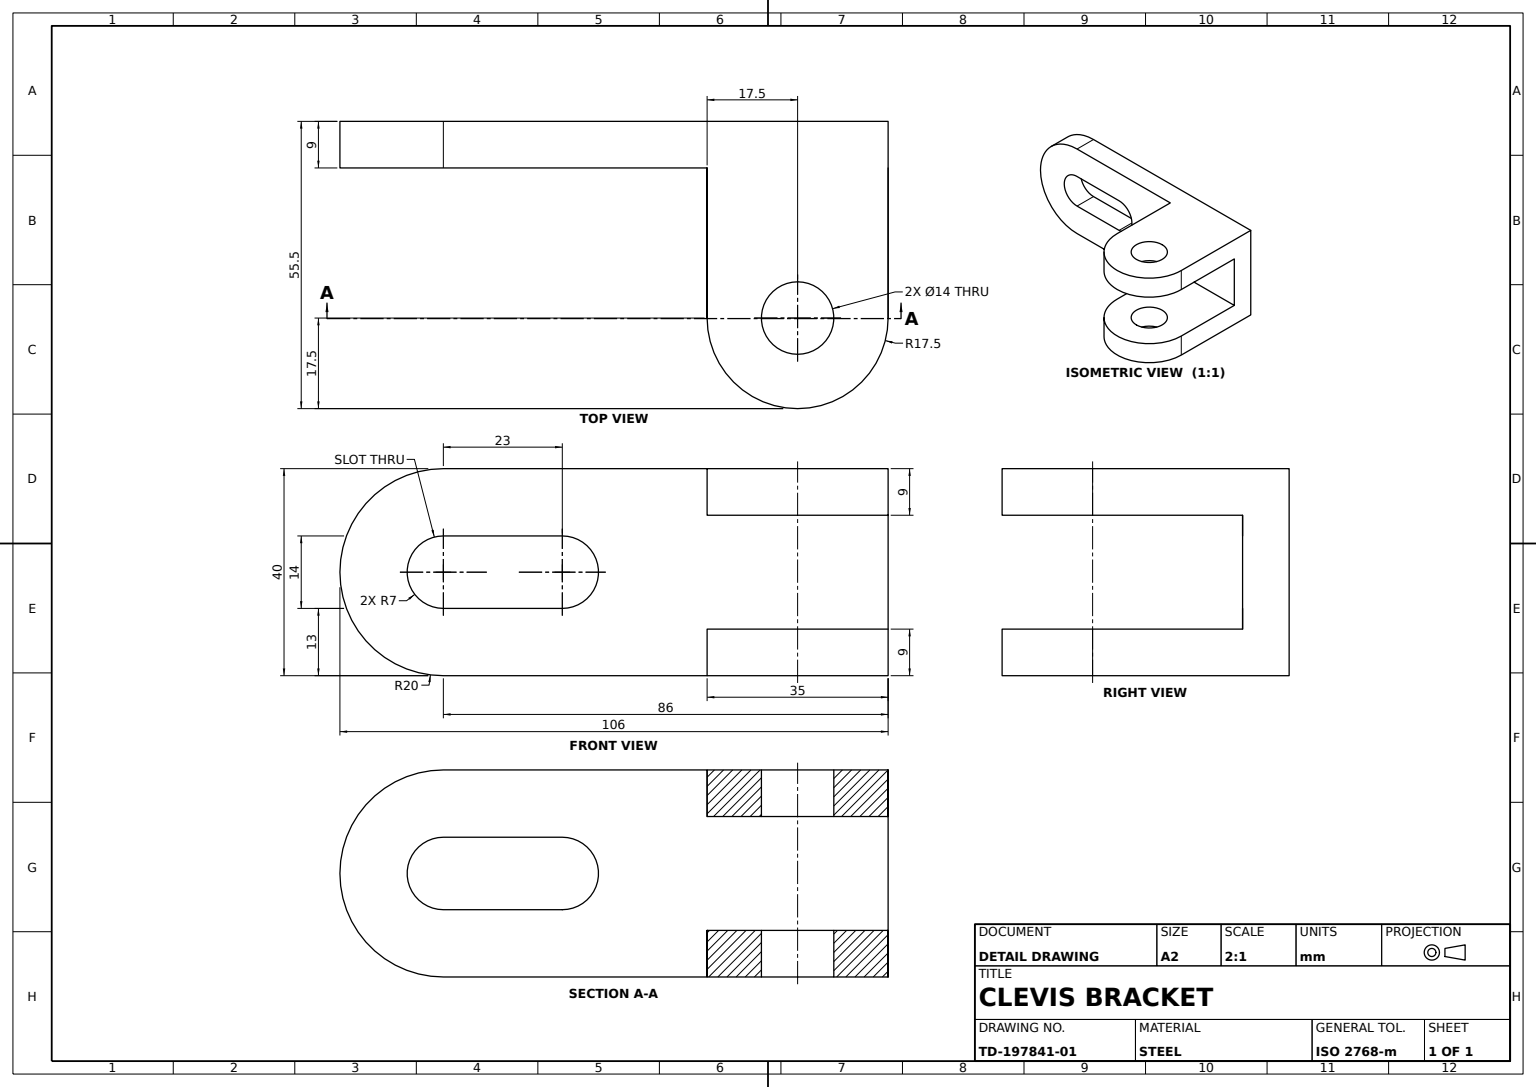
SolidWorks part; units mm, degrees
material "Plain Carbon Steel"
ref_plane "Front Plane" through (0, 0, 0) normal (1, 0, 0) x (0, 1, 0)
ref_plane "Top Plane" through (0, 0, 0) normal (0, 0, 1) x (0, 1, 0)
ref_plane "Right Plane" through (0, 0, 0) normal (0, 1, 0) x (-1, 0, 0)
sketch "Base Plate Sketch" plane through (0, 0, 0) normal (0, 0, 1) x (-1, 0, 0)
  line L1 (0, 0) -> (86, 0)
  line L2 (0, 0) -> (0, 40)
  line L3 (0, 40) -> (86, 40)
  arc A0 (86, 40) -> (86, 0) centre (86, 20) cw
  dimension "D1" = 20
  dimension "D2" = 86
extrude "Base Plate" add sketch "Base Plate Sketch" along normal blind 9
sketch "Base Slot Sketch" plane through (0, 0, 0) normal (0, 0, -1) x (1, 0, 0)
  line L0 (-86, 20) -> (-63, 20) construction
  line L1 (-86, 27) -> (-63, 27)
  line L2 (-86, 13) -> (-63, 13)
  arc A0 (-86, 27) -> (-86, 13) centre (-86, 20) ccw
  arc A1 (-63, 13) -> (-63, 27) centre (-63, 20) ccw
  point P3 (-74.5, 20)
  dimension "D1" = 14
  dimension "D2" = 23
extrude "Base Slot" cut sketch "Base Slot Sketch" against normal blind 28
sketch "Clevis Ear 1 Sketch" plane through (0, -40, 0) normal (0, -1, 0) x (1, 0, 0)
  line L0 (0, 9) -> (0, 38)
  line L1 (-35, 38) -> (-35, 9)
  line L2 (-86, 9) -> (0, 9) construction
  line L3 (-35, 9) -> (0, 9)
  line L4 (-86, 0) -> (0, 0) construction
  arc A0 (0, 38) -> (-35, 38) centre (-17.5, 38) ccw
  dimension "D1" = 17.5
  dimension "D2" = 38
extrude "Clevis Ear 1" add sketch "Clevis Ear 1 Sketch" against normal blind 9 contours L1 L3 L0 A0
sketch "Clevis Ear 2 Sketch" plane through (0, 0, 0) normal (0, 1, 0) x (-1, 0, 0)
  line L0 (0, 9) -> (0, 38)
  line L1 (35, 38) -> (35, 9)
  line L2 (35, 9) -> (0, 9)
  arc A0 (0, 38) -> (35, 38) centre (17.5, 38) cw
extrude "Clevis Ear 2" add sketch "Clevis Ear 2 Sketch" against normal blind 9
sketch "Pin Hole Sketch" plane through (0, 0, 0) normal (0, 1, 0) x (-1, 0, 0)
  line L0 (17.5, 55.5) -> (17.5, 0) construction
  line L1 (0, 0) -> (86, 0) construction
  circle A0 centre (17.5, 38) radius 7
  arc A1 (35, 38) -> (0, 38) centre (17.5, 38) ccw construction
  dimension "D1" = 14
  dimension "D2" = 38
extrude "Pin Hole" cut sketch "Pin Hole Sketch" against normal blind 80
